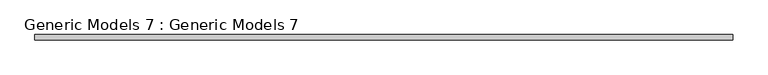
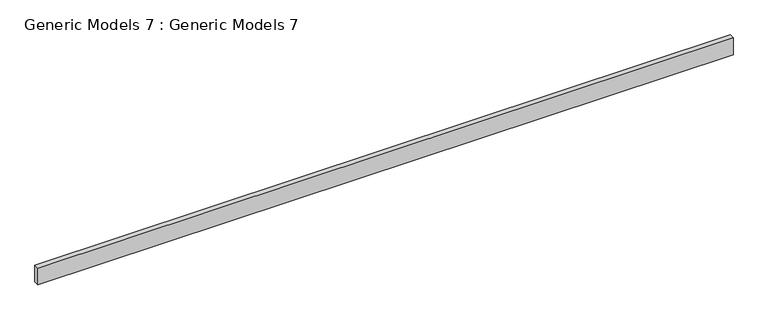
"""IFC4 building model written with IfcOpenShell, lengths in millimetres: proxy geometry, Generic Models 7 : Generic Models 7."""

from ifc_helpers import new_model, si_unit, frame, origin, place, context, project, spatial, polyline, outline, extrude, source, transform, mapped, element, save


def generic_models_7_generic_models_7_d0c4d58f(model_context):
    return source(origin(), model_context, "Body", "SweptSolid", [
        extrude(outline(polyline([(12604.4370151, -3746.0004242), (12604.4370151, -3911.1714442), (-8934.7629849, -3911.1714442), (-8934.7629849, -3746.0004242), (12604.4370151, -3746.0004242)])), frame((0.0, 0.0, 16040.5989528), z_axis=(0.0, 0.0, 1.0), x_axis=(1.0, 0.0, 0.0)), (0.0, 0.0, 1.0), 551.8243167),
    ])


if __name__ == "__main__":
    model = new_model("IFC4")
    model_context = context("Model", 3, world=origin())
    ifc_project = project(units=[si_unit("LENGTHUNIT", "METRE", prefix="MILLI")], contexts=[model_context])
    site = spatial("IfcSite", under=ifc_project)
    building = spatial("IfcBuilding", under=site)
    placement = place(None, origin())
    generic_models_7_generic_models_7_shape = generic_models_7_generic_models_7_d0c4d58f(model_context)
    element("IfcBuildingElementProxy", 1, Name="Generic Models 7 : Generic Models 7", ObjectType="Generic Models 7 : Generic Models 7", at=placement, inside=building, context=model_context, shape_type="MappedRepresentation", body=[
        mapped(generic_models_7_generic_models_7_shape, transform((0.0, 0.0, 0.0), x_axis=(1.0, 0.0, 0.0), y_axis=(0.0, 1.0, 0.0), z_axis=(0.0, 0.0, 1.0))),
    ])
    save(model, "model.ifc")
